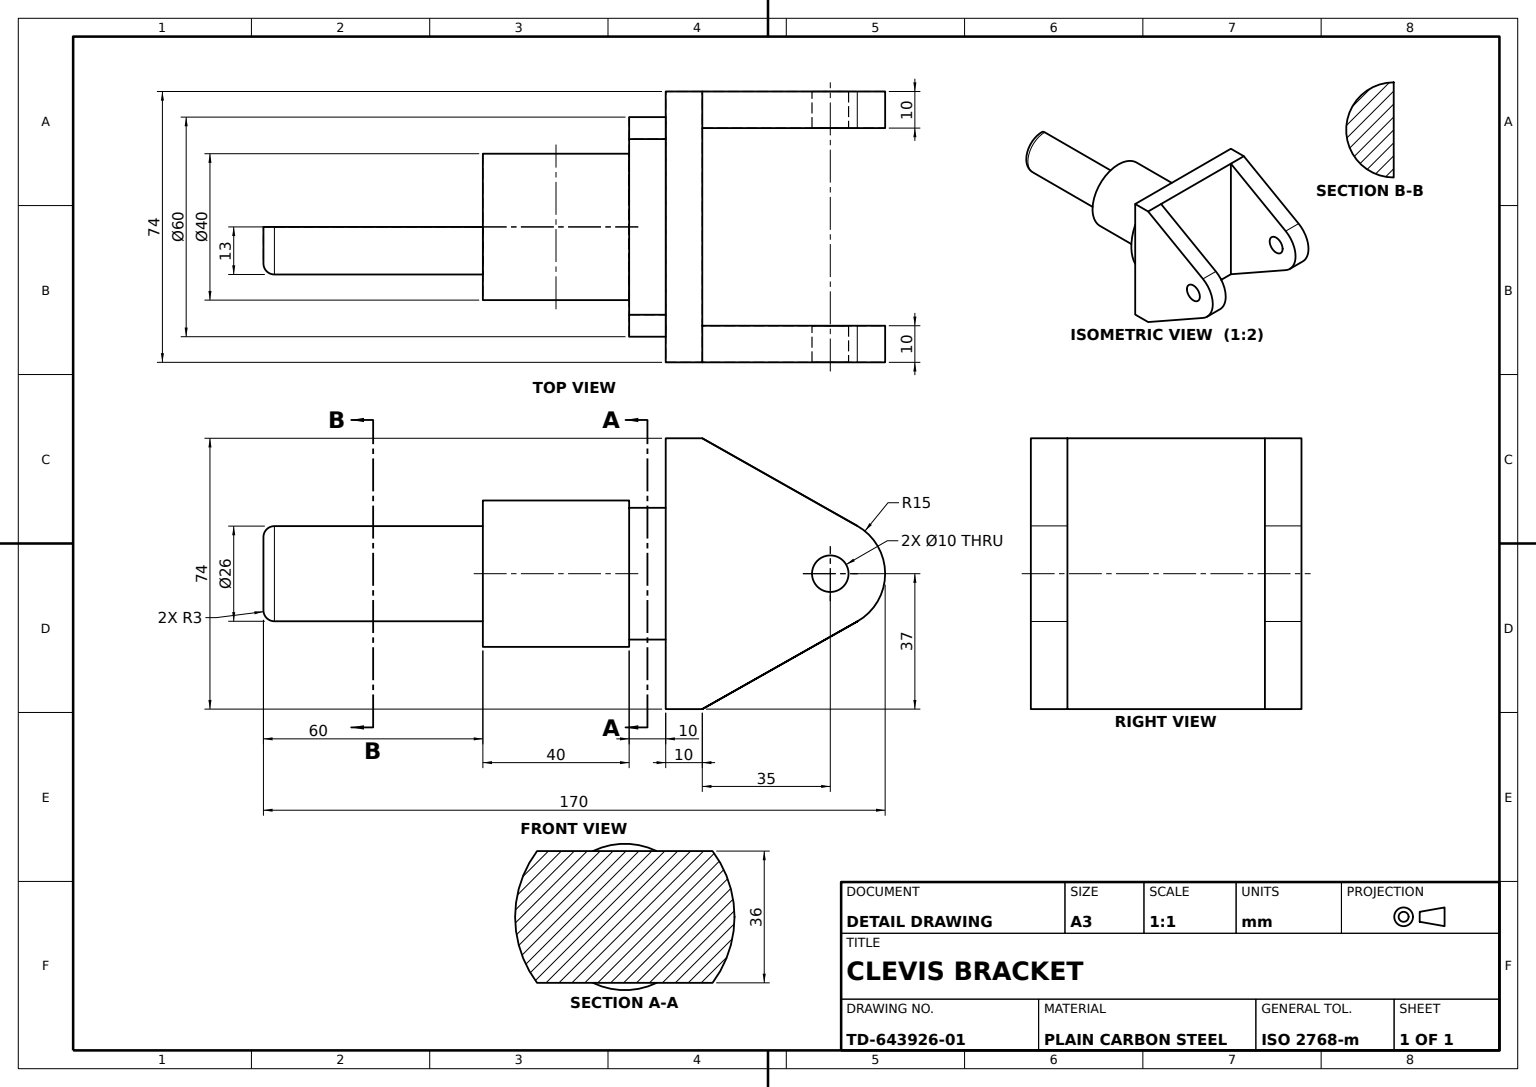
SolidWorks part; units mm, degrees
material "Plain Carbon Steel"
ref_plane "Front Plane" through (0, 0, 0) normal (0, 0, 1) x (1, 0, 0)
ref_plane "Top Plane" through (0, 0, 0) normal (0, 1, 0) x (1, 0, 0)
ref_plane "Right Plane" through (0, 0, 0) normal (1, 0, 0) x (0, 0, -1)
sketch "Base Disc Sketch Ø60" plane through (0, 0, 0) normal (0, 0, 1) x (1, 0, 0)
  circle A0 centre (0, 0) radius 30
  dimension "D1" = 60
extrude "Base Disc Ø60" add sketch "Base Disc Sketch Ø60" along normal blind 10
sketch "Base Profile Cut Sketch" plane through (0, 0, 10) normal (0, 0, 1) x (1, 0, 0)
  line L0 (0, 0) -> (0, 12) construction
  line L1 (0, 0) -> (0, -12) construction
  line L2 (0, 30) -> (0, 18) construction
  line L3 (0, 18) -> (-24, 18)
  line L4 (0, 18) -> (24, 18)
  line L5 (0, 12) -> (0, 30) construction
  line L6 (0, -12) -> (0, -30) construction
  line L7 (0, -30) -> (0, -18) construction
  line L8 (0, -18) -> (24, -18)
  line L9 (0, -18) -> (-24, -18)
  circle A0 centre (0, 0) radius 30 construction
  arc A1 (-24, -18) -> (24, -18) centre (0, 0) ccw
  arc A2 (24, 18) -> (-24, 18) centre (0, 0) ccw
  dimension "D1" = 30
  dimension "D2" = 24
extrude "Base Profile Cut" cut sketch "Base Profile Cut Sketch" against normal blind 10
sketch "Collar Sketch Ø40" plane through (0, 0, 10) normal (0, 0, 1) x (1, 0, 0)
  circle A0 centre (0, 0) radius 20
  dimension "D1" = 40
extrude "Collar Ø40" add sketch "Collar Sketch Ø40" along normal blind 40
sketch "Shaft Sketch Ø26" plane through (0, 0, 50) normal (0, 0, 1) x (1, 0, 0)
  circle A0 centre (0, 0) radius 13
  dimension "D1" = 26
extrude "Shaft Ø26" add sketch "Shaft Sketch Ø26" along normal blind 60
fillet "Shaft End Fillet R3" radius 3 1 edges at (13, 0, 110)
ref_plane "Shaft Flat Plane" through (0, 0, 0) normal (1, 0, 0) x (0, 0, -1)
sketch "Shaft Flat Sketch" plane through (0, 0, 0) normal (1, 0, 0) x (0, 0, -1)
  line L0 (-107, 20.0223) -> (-120.8287, 20.0223)
  line L1 (-50, 20.0223) -> (-107, 20.0223)
  line L2 (-50, 20.0223) -> (-50, -20.0223)
  line L3 (-50, -20.0223) -> (-107, -20.0223)
  line L7 (-120.8287, 20.0223) -> (-120.8287, -20.0223)
  line L8 (-120.8287, -20.0223) -> (-107, -20.0223)
  point P0 (-78.5, 0)
  dimension "D1" = 40.0446
  dimension "D2" = 20.0223
  dimension "D3" = 50
  dimension "D4" = 57
  dimension "D5" = 13.8287
  dimension "D6" = 78.5
extrude "Shaft Flat Cut" cut sketch "Shaft Flat Sketch" against normal blind 30
sketch "Mounting Flange Sketch 74" plane through (0, 0, 0) normal (0, 0, -1) x (-1, 0, 0)
  line L1 (-37, 37) -> (37, 37)
  line L2 (-37, 37) -> (-37, -37)
  line L3 (-37, -37) -> (37, -37)
  line L4 (37, 37) -> (37, -37)
  line L5 (-37, 37) -> (37, -37) construction
  line L6 (-37, -37) -> (37, 37) construction
  point P0 (0, 0)
  dimension "D1" = 74
extrude "Mounting Flange 74" add sketch "Mounting Flange Sketch 74" along normal blind 10
ref_plane "Mounting Ear Plane" through (37, 0, 0) normal (1, 0, 0) x (0, 0, -1)
sketch "Mounting Ear Sketch" plane through (37, 0, 0) normal (1, 0, 0) x (0, 0, -1)
  line L0 (10, -37) -> (10, 37) construction
  line L1 (10, 37) -> (52.3779, 13.0601)
  line L2 (10, -37) -> (52.3779, -13.0601)
  line L3 (10, 37) -> (10, -37)
  arc A0 (52.3779, -13.0601) -> (52.3779, 13.0601) centre (45, 0) ccw
  dimension "D1" = 30
  dimension "D2" = 35
  dimension "D3" = 45
extrude "Mounting Ear" add sketch "Mounting Ear Sketch" against normal blind 10
ref_plane "Ear Mirror Plane" through (0, 0, 0) normal (1, 0, 0) x (0, 0, -1)
mirror "Mounting Ear Mirror" about plane through (0, 0, 0) normal (1, 0, 0) of "Mounting Ear"
sketch "Ear Hole Sketch Ø10" plane through (37, 0, 0) normal (1, 0, 0) x (0, 0, -1)
  circle A0 centre (45, 0) radius 5
  dimension "D1" = 10
extrude "Ear Hole Ø10" cut sketch "Ear Hole Sketch Ø10" against normal through all
